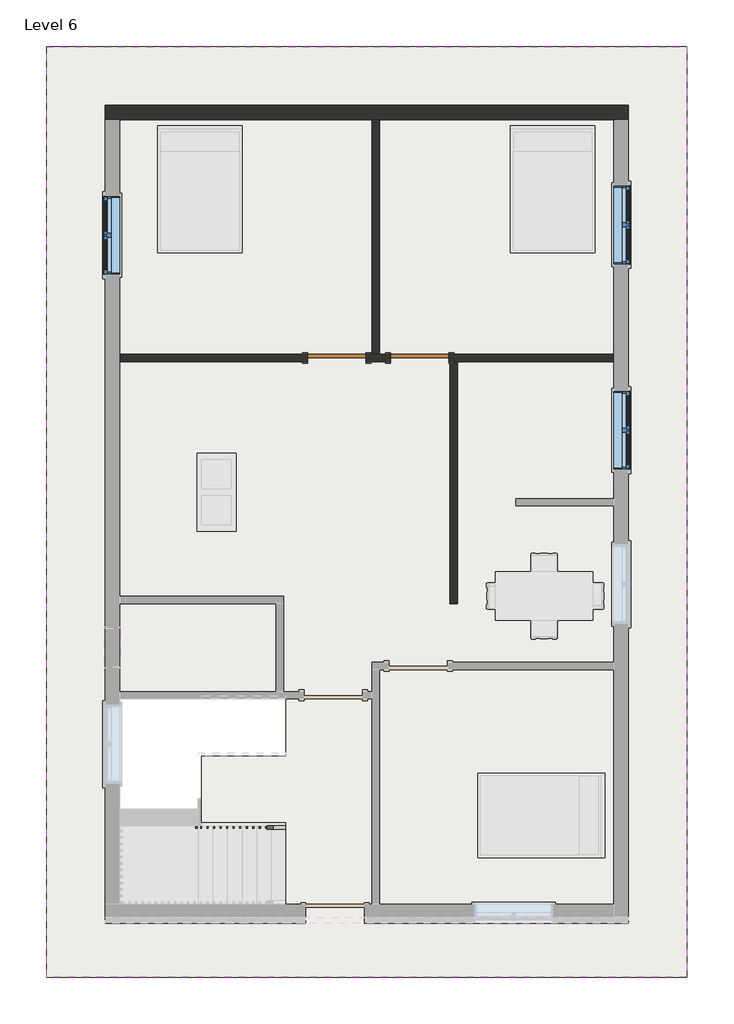
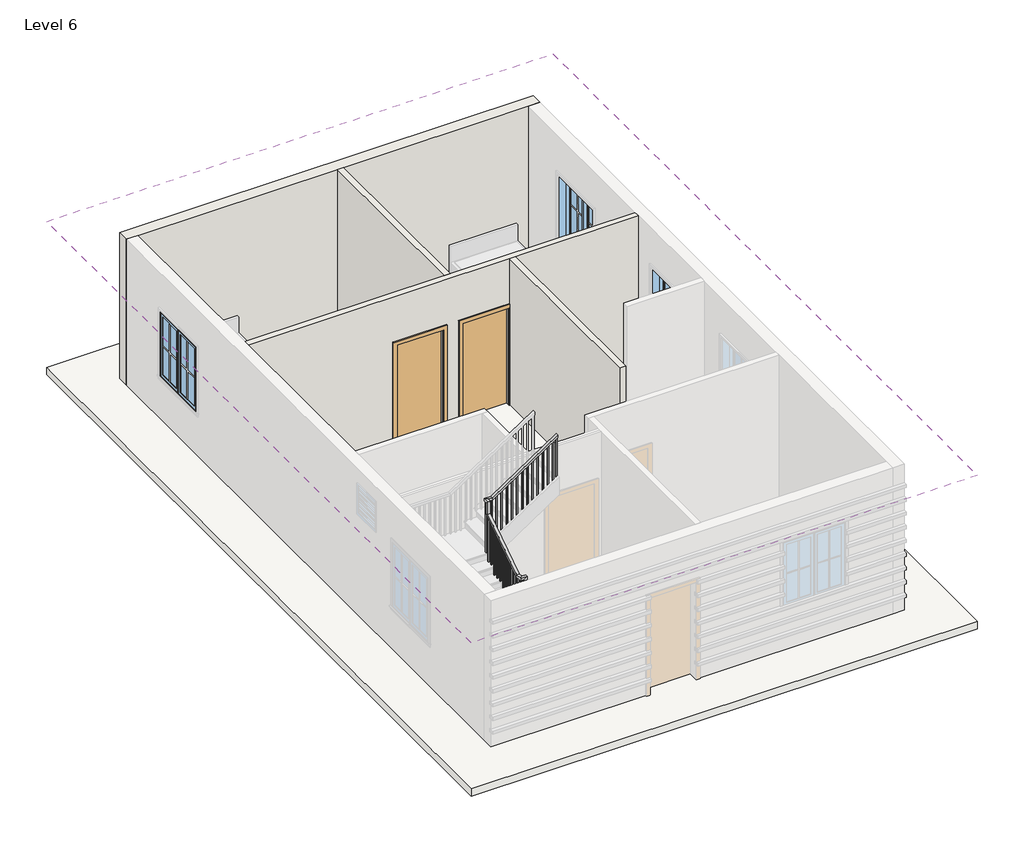
# One storey, part 2 of 3: 4 walls, 3 windows, 2 doors, 2 roofs, 1 railing.
"""IFC4 building model written with IfcOpenShell, lengths in millimetres."""

from ifc_helpers import new_model, si_unit, frame, origin, place, context, project, spatial, polyline, outline, extrude, faceted_brep, transform, mapped, element, save
from components import single_flush_door_3_17d80c48, single_flush_door_3_5e62189b, window_casement_double_window_4_576b2d2c

model = new_model("IFC4")

# Units and contexts
model_context = context("Model", 3, world=origin())
ifc_project = project(units=[si_unit("LENGTHUNIT", "METRE", prefix="MILLI")], contexts=[model_context])

# Site, building, storey
site = spatial("IfcSite", under=ifc_project)
building = spatial("IfcBuilding", under=site)
storey = spatial("IfcBuildingStorey", under=building, Name="Level 6", Elevation=15849.6)

# Doors
placement = place(None, origin())
single_flush_door_3_shape = single_flush_door_3_17d80c48(model_context)
element("IfcDoor", 1, ObjectType="Single-Flush : DOOR 3'", at=placement, inside=storey, context=model_context, shape_type="MappedRepresentation", body=[
    mapped(single_flush_door_3_shape, transform((-1721.4617403, 2133.1073441, 15849.6), x_axis=(1.0, 0.0, 0.0), y_axis=(0.0, 1.0, 0.0), z_axis=(0.0, 0.0, 1.0))),
])
single_flush_door_3_2_shape = single_flush_door_3_5e62189b(model_context)
element("IfcDoor", 2, ObjectType="Single-Flush : DOOR 3'", at=placement, inside=storey, context=model_context, shape_type="MappedRepresentation", body=[
    mapped(single_flush_door_3_2_shape, transform((-426.0617403, 2133.1073441, 15849.6), x_axis=(-1.0, 0.0, 0.0), y_axis=(0.0, -1.0, 0.0), z_axis=(0.0, 0.0, 1.0))),
])

# Railing
element("IfcRailing", 3, ObjectType="Handrail - Rectangular", at=placement, inside=storey, context=model_context, shape_type="SolidModel", body=[
    faceted_brep([(-2515.2117403, -5213.8426559, 16916.4), (-2515.2117403, -5213.8426559, 16855.3459984), (-2515.2117403, -5163.0426559, 16855.3459984), (-2515.2117403, -5163.0426559, 16916.4), (-3810.6117403, -5213.8426559, 17780.0), (-3861.4117403, -5213.8426559, 17752.8126651), (-3861.4117403, -5163.0426559, 17752.8126651), (-3810.6117403, -5163.0426559, 17780.0), (-3810.6117403, -5213.8426559, 18034.0), (-3861.4117403, -5213.8426559, 17983.2), (-3861.4117403, -5163.0426559, 17983.2), (-3810.6117403, -5163.0426559, 18034.0), (-3937.6117403, -5213.8426559, 18034.0), (-3937.6117403, -5213.8426559, 17983.2), (-3886.8117403, -5163.0426559, 17983.2), (-3886.8117403, -5163.0426559, 18034.0), (-3937.6117403, -5086.8426559, 18034.0), (-3937.6117403, -5071.4616535, 17983.2), (-3886.8117403, -5071.4616535, 17983.2), (-3886.8117403, -5086.8426559, 18034.0), (-3937.6117403, -4096.2426559, 18694.4), (-3937.6117403, -4045.4426559, 18667.2126651), (-3886.8117403, -4045.4426559, 18667.2126651), (-3886.8117403, -4096.2426559, 18694.4), (-3937.6117403, -4096.2426559, 18948.4), (-3937.6117403, -4045.4426559, 18897.6), (-3886.8117403, -4045.4426559, 18897.6), (-3886.8117403, -4096.2426559, 18948.4), (-3937.6117403, -3969.2426559, 18948.4), (-3937.6117403, -3969.2426559, 18897.6), (-3886.8117403, -4020.0426559, 18897.6), (-3886.8117403, -4020.0426559, 18948.4), (-3810.6117403, -3969.2426559, 18948.4), (-3795.2307379, -3969.2426559, 18897.6), (-3795.2307379, -4020.0426559, 18897.6), (-3810.6117403, -4020.0426559, 18948.4), (-2515.2117403, -3969.2426559, 19812.0), (-2515.2117403, -4020.0426559, 19812.0), (-2515.2117403, -4020.0426559, 19750.9459984), (-2515.2117403, -3969.2426559, 19750.9459984)], [[[0, 1, 2, 3]], [[1, 0, 4, 5]], [[2, 1, 5, 6]], [[3, 2, 6, 7]], [[0, 3, 7, 4]], [[5, 4, 8, 9]], [[6, 5, 9, 10]], [[7, 6, 10, 11]], [[4, 7, 11, 8]], [[9, 8, 12, 13]], [[10, 9, 13, 14]], [[11, 10, 14, 15]], [[8, 11, 15, 12]], [[13, 12, 16, 17]], [[14, 13, 17, 18]], [[15, 14, 18, 19]], [[12, 15, 19, 16]], [[17, 16, 20, 21]], [[18, 17, 21, 22]], [[19, 18, 22, 23]], [[16, 19, 23, 20]], [[21, 20, 24, 25]], [[22, 21, 25, 26]], [[23, 22, 26, 27]], [[20, 23, 27, 24]], [[25, 24, 28, 29]], [[26, 25, 29, 30]], [[27, 26, 30, 31]], [[24, 27, 31, 28]], [[29, 28, 32, 33]], [[30, 29, 33, 34]], [[31, 30, 34, 35]], [[28, 31, 35, 32]], [[36, 37, 38, 39]], [[33, 32, 36, 39]], [[34, 33, 39, 38]], [[35, 34, 38, 37]], [[32, 35, 37, 36]]]),
    extrude(outline(polyline([(19706.4959984, -2581.8867403), (19693.7959984, -2600.9367403), (18745.2, -2600.9367403), (18745.2, -2581.8867403), (19706.4959984, -2581.8867403)])), frame((0.0, -4004.1676559, 0.0), z_axis=(0.0, 1.0, 0.0), x_axis=(0.0, 0.0, 1.0)), (0.0, 0.0, 1.0), 19.05),
    extrude(outline(polyline([(19638.7626651, -2683.4867403), (19626.0626651, -2702.5367403), (18745.2, -2702.5367403), (18745.2, -2683.4867403), (19638.7626651, -2683.4867403)])), frame((0.0, -4004.1676559, 0.0), z_axis=(0.0, 1.0, 0.0), x_axis=(0.0, 0.0, 1.0)), (0.0, 0.0, 1.0), 19.05),
    extrude(outline(polyline([(19571.0293317, -2785.0867403), (19558.3293317, -2804.1367403), (18592.8, -2804.1367403), (18592.8, -2785.0867403), (19571.0293317, -2785.0867403)])), frame((0.0, -4004.1676559, 0.0), z_axis=(0.0, 1.0, 0.0), x_axis=(0.0, 0.0, 1.0)), (0.0, 0.0, 1.0), 19.05),
    extrude(outline(polyline([(19503.2959984, -2886.6867403), (19490.5959984, -2905.7367403), (18592.8, -2905.7367403), (18592.8, -2886.6867403), (19503.2959984, -2886.6867403)])), frame((0.0, -4004.1676559, 0.0), z_axis=(0.0, 1.0, 0.0), x_axis=(0.0, 0.0, 1.0)), (0.0, 0.0, 1.0), 19.05),
    extrude(outline(polyline([(19435.5626651, -2988.2867403), (19422.8626651, -3007.3367403), (18440.4, -3007.3367403), (18440.4, -2988.2867403), (19435.5626651, -2988.2867403)])), frame((0.0, -4004.1676559, 0.0), z_axis=(0.0, 1.0, 0.0), x_axis=(0.0, 0.0, 1.0)), (0.0, 0.0, 1.0), 19.05),
    extrude(outline(polyline([(19367.8293317, -3089.8867403), (19355.1293317, -3108.9367403), (18440.4, -3108.9367403), (18440.4, -3089.8867403), (19367.8293317, -3089.8867403)])), frame((0.0, -4004.1676559, 0.0), z_axis=(0.0, 1.0, 0.0), x_axis=(0.0, 0.0, 1.0)), (0.0, 0.0, 1.0), 19.05),
    extrude(outline(polyline([(19300.0959984, -3191.4867403), (19287.3959984, -3210.5367403), (18440.4, -3210.5367403), (18440.4, -3191.4867403), (19300.0959984, -3191.4867403)])), frame((0.0, -4004.1676559, 0.0), z_axis=(0.0, 1.0, 0.0), x_axis=(0.0, 0.0, 1.0)), (0.0, 0.0, 1.0), 19.05),
    extrude(outline(polyline([(19232.3626651, -3293.0867403), (19219.6626651, -3312.1367403), (18288.0, -3312.1367403), (18288.0, -3293.0867403), (19232.3626651, -3293.0867403)])), frame((0.0, -4004.1676559, 0.0), z_axis=(0.0, 1.0, 0.0), x_axis=(0.0, 0.0, 1.0)), (0.0, 0.0, 1.0), 19.05),
    extrude(outline(polyline([(19164.6293317, -3394.6867403), (19151.9293317, -3413.7367403), (18288.0, -3413.7367403), (18288.0, -3394.6867403), (19164.6293317, -3394.6867403)])), frame((0.0, -4004.1676559, 0.0), z_axis=(0.0, 1.0, 0.0), x_axis=(0.0, 0.0, 1.0)), (0.0, 0.0, 1.0), 19.05),
    extrude(outline(polyline([(19096.8959984, -3496.2867403), (19084.1959984, -3515.3367403), (18135.6, -3515.3367403), (18135.6, -3496.2867403), (19096.8959984, -3496.2867403)])), frame((0.0, -4004.1676559, 0.0), z_axis=(0.0, 1.0, 0.0), x_axis=(0.0, 0.0, 1.0)), (0.0, 0.0, 1.0), 19.05),
    extrude(outline(polyline([(19029.1626651, -3597.8867403), (19016.4626651, -3616.9367403), (18135.6, -3616.9367403), (18135.6, -3597.8867403), (19029.1626651, -3597.8867403)])), frame((0.0, -4004.1676559, 0.0), z_axis=(0.0, 1.0, 0.0), x_axis=(0.0, 0.0, 1.0)), (0.0, 0.0, 1.0), 19.05),
    extrude(outline(polyline([(18961.4293317, -3699.4867403), (18948.7293317, -3718.5367403), (17983.2, -3718.5367403), (17983.2, -3699.4867403), (18961.4293317, -3699.4867403)])), frame((0.0, -4004.1676559, 0.0), z_axis=(0.0, 1.0, 0.0), x_axis=(0.0, 0.0, 1.0)), (0.0, 0.0, 1.0), 19.05),
    extrude(outline(polyline([(18893.6959984, -3801.0867403), (18880.9959984, -3820.1367403), (17983.2, -3820.1367403), (17983.2, -3801.0867403), (18893.6959984, -3801.0867403)])), frame((0.0, -4004.1676559, 0.0), z_axis=(0.0, 1.0, 0.0), x_axis=(0.0, 0.0, 1.0)), (0.0, 0.0, 1.0), 19.05),
    extrude(outline(polyline([(-3902.6867403, -4080.3676559), (-3921.7367403, -4080.3676559), (-3921.7367403, -4061.3176559), (-3902.6867403, -4061.3176559), (-3902.6867403, -4080.3676559)])), frame((0.0, 0.0, 17678.4), z_axis=(0.0, 0.0, 1.0), x_axis=(1.0, 0.0, 0.0)), (0.0, 0.0, 1.0), 1219.2),
    extrude(outline(polyline([(-4181.9676559, 18576.1959984), (-4162.9176559, 18588.8959984), (-4162.9176559, 17678.4), (-4181.9676559, 17678.4), (-4181.9676559, 18576.1959984)])), frame((-3921.7367403, 0.0, 0.0), z_axis=(1.0, 0.0, 0.0), x_axis=(0.0, 1.0, 0.0)), (0.0, 0.0, 1.0), 19.05),
    extrude(outline(polyline([(-4283.5676559, 18508.4626651), (-4264.5176559, 18521.1626651), (-4264.5176559, 17526.0), (-4283.5676559, 17526.0), (-4283.5676559, 18508.4626651)])), frame((-3921.7367403, 0.0, 0.0), z_axis=(1.0, 0.0, 0.0), x_axis=(0.0, 1.0, 0.0)), (0.0, 0.0, 1.0), 19.05),
    extrude(outline(polyline([(-4385.1676559, 18440.7293317), (-4366.1176559, 18453.4293317), (-4366.1176559, 17526.0), (-4385.1676559, 17526.0), (-4385.1676559, 18440.7293317)])), frame((-3921.7367403, 0.0, 0.0), z_axis=(1.0, 0.0, 0.0), x_axis=(0.0, 1.0, 0.0)), (0.0, 0.0, 1.0), 19.05),
    extrude(outline(polyline([(-4486.7676559, 18372.9959984), (-4467.7176559, 18385.6959984), (-4467.7176559, 17526.0), (-4486.7676559, 17526.0), (-4486.7676559, 18372.9959984)])), frame((-3921.7367403, 0.0, 0.0), z_axis=(1.0, 0.0, 0.0), x_axis=(0.0, 1.0, 0.0)), (0.0, 0.0, 1.0), 19.05),
    extrude(outline(polyline([(-4588.3676559, 18305.2626651), (-4569.3176559, 18317.9626651), (-4569.3176559, 17373.6), (-4588.3676559, 17373.6), (-4588.3676559, 18305.2626651)])), frame((-3921.7367403, 0.0, 0.0), z_axis=(1.0, 0.0, 0.0), x_axis=(0.0, 1.0, 0.0)), (0.0, 0.0, 1.0), 19.05),
    extrude(outline(polyline([(-4689.9676559, 18237.5293317), (-4670.9176559, 18250.2293317), (-4670.9176559, 17373.6), (-4689.9676559, 17373.6), (-4689.9676559, 18237.5293317)])), frame((-3921.7367403, 0.0, 0.0), z_axis=(1.0, 0.0, 0.0), x_axis=(0.0, 1.0, 0.0)), (0.0, 0.0, 1.0), 19.05),
    extrude(outline(polyline([(-4791.5676559, 18169.7959984), (-4772.5176559, 18182.4959984), (-4772.5176559, 17221.2), (-4791.5676559, 17221.2), (-4791.5676559, 18169.7959984)])), frame((-3921.7367403, 0.0, 0.0), z_axis=(1.0, 0.0, 0.0), x_axis=(0.0, 1.0, 0.0)), (0.0, 0.0, 1.0), 19.05),
    extrude(outline(polyline([(-4893.1676559, 18102.0626651), (-4874.1176559, 18114.7626651), (-4874.1176559, 17221.2), (-4893.1676559, 17221.2), (-4893.1676559, 18102.0626651)])), frame((-3921.7367403, 0.0, 0.0), z_axis=(1.0, 0.0, 0.0), x_axis=(0.0, 1.0, 0.0)), (0.0, 0.0, 1.0), 19.05),
    extrude(outline(polyline([(-4994.7676559, 18034.3293317), (-4975.7176559, 18047.0293317), (-4975.7176559, 17068.8), (-4994.7676559, 17068.8), (-4994.7676559, 18034.3293317)])), frame((-3921.7367403, 0.0, 0.0), z_axis=(1.0, 0.0, 0.0), x_axis=(0.0, 1.0, 0.0)), (0.0, 0.0, 1.0), 19.05),
    extrude(outline(polyline([(-5096.3676559, 17966.5959984), (-5077.3176559, 17979.2959984), (-5077.3176559, 17068.8), (-5096.3676559, 17068.8), (-5096.3676559, 17966.5959984)])), frame((-3921.7367403, 0.0, 0.0), z_axis=(1.0, 0.0, 0.0), x_axis=(0.0, 1.0, 0.0)), (0.0, 0.0, 1.0), 19.05),
    extrude(outline(polyline([(-3826.4867403, -5178.9176559), (-3826.4867403, -5197.9676559), (-3845.5367403, -5197.9676559), (-3845.5367403, -5178.9176559), (-3826.4867403, -5178.9176559)])), frame((0.0, 0.0, 16764.0), z_axis=(0.0, 0.0, 1.0), x_axis=(1.0, 0.0, 0.0)), (0.0, 0.0, 1.0), 1219.2),
    extrude(outline(polyline([(17661.7959984, -3724.8867403), (17674.4959984, -3743.9367403), (16764.0, -3743.9367403), (16764.0, -3724.8867403), (17661.7959984, -3724.8867403)])), frame((0.0, -5197.9676559, 0.0), z_axis=(0.0, 1.0, 0.0), x_axis=(0.0, 0.0, 1.0)), (0.0, 0.0, 1.0), 19.05),
    extrude(outline(polyline([(17594.0626651, -3623.2867403), (17606.7626651, -3642.3367403), (16611.6, -3642.3367403), (16611.6, -3623.2867403), (17594.0626651, -3623.2867403)])), frame((0.0, -5197.9676559, 0.0), z_axis=(0.0, 1.0, 0.0), x_axis=(0.0, 0.0, 1.0)), (0.0, 0.0, 1.0), 19.05),
    extrude(outline(polyline([(17526.3293317, -3521.6867403), (17539.0293317, -3540.7367403), (16611.6, -3540.7367403), (16611.6, -3521.6867403), (17526.3293317, -3521.6867403)])), frame((0.0, -5197.9676559, 0.0), z_axis=(0.0, 1.0, 0.0), x_axis=(0.0, 0.0, 1.0)), (0.0, 0.0, 1.0), 19.05),
    extrude(outline(polyline([(17458.5959984, -3420.0867403), (17471.2959984, -3439.1367403), (16611.6, -3439.1367403), (16611.6, -3420.0867403), (17458.5959984, -3420.0867403)])), frame((0.0, -5197.9676559, 0.0), z_axis=(0.0, 1.0, 0.0), x_axis=(0.0, 0.0, 1.0)), (0.0, 0.0, 1.0), 19.05),
    extrude(outline(polyline([(17390.8626651, -3318.4867403), (17403.5626651, -3337.5367403), (16459.2, -3337.5367403), (16459.2, -3318.4867403), (17390.8626651, -3318.4867403)])), frame((0.0, -5197.9676559, 0.0), z_axis=(0.0, 1.0, 0.0), x_axis=(0.0, 0.0, 1.0)), (0.0, 0.0, 1.0), 19.05),
    extrude(outline(polyline([(17323.1293317, -3216.8867403), (17335.8293317, -3235.9367403), (16459.2, -3235.9367403), (16459.2, -3216.8867403), (17323.1293317, -3216.8867403)])), frame((0.0, -5197.9676559, 0.0), z_axis=(0.0, 1.0, 0.0), x_axis=(0.0, 0.0, 1.0)), (0.0, 0.0, 1.0), 19.05),
    extrude(outline(polyline([(17255.3959984, -3115.2867403), (17268.0959984, -3134.3367403), (16306.8, -3134.3367403), (16306.8, -3115.2867403), (17255.3959984, -3115.2867403)])), frame((0.0, -5197.9676559, 0.0), z_axis=(0.0, 1.0, 0.0), x_axis=(0.0, 0.0, 1.0)), (0.0, 0.0, 1.0), 19.05),
    extrude(outline(polyline([(17187.6626651, -3013.6867403), (17200.3626651, -3032.7367403), (16306.8, -3032.7367403), (16306.8, -3013.6867403), (17187.6626651, -3013.6867403)])), frame((0.0, -5197.9676559, 0.0), z_axis=(0.0, 1.0, 0.0), x_axis=(0.0, 0.0, 1.0)), (0.0, 0.0, 1.0), 19.05),
    extrude(outline(polyline([(17119.9293317, -2912.0867403), (17132.6293317, -2931.1367403), (16154.4, -2931.1367403), (16154.4, -2912.0867403), (17119.9293317, -2912.0867403)])), frame((0.0, -5197.9676559, 0.0), z_axis=(0.0, 1.0, 0.0), x_axis=(0.0, 0.0, 1.0)), (0.0, 0.0, 1.0), 19.05),
    extrude(outline(polyline([(17052.1959984, -2810.4867403), (17064.8959984, -2829.5367403), (16154.4, -2829.5367403), (16154.4, -2810.4867403), (17052.1959984, -2810.4867403)])), frame((0.0, -5197.9676559, 0.0), z_axis=(0.0, 1.0, 0.0), x_axis=(0.0, 0.0, 1.0)), (0.0, 0.0, 1.0), 19.05),
    extrude(outline(polyline([(16984.4626651, -2708.8867403), (16997.1626651, -2727.9367403), (16002.0, -2727.9367403), (16002.0, -2708.8867403), (16984.4626651, -2708.8867403)])), frame((0.0, -5197.9676559, 0.0), z_axis=(0.0, 1.0, 0.0), x_axis=(0.0, 0.0, 1.0)), (0.0, 0.0, 1.0), 19.05),
    extrude(outline(polyline([(16916.7293317, -2607.2867403), (16929.4293317, -2626.3367403), (16002.0, -2626.3367403), (16002.0, -2607.2867403), (16916.7293317, -2607.2867403)])), frame((0.0, -5197.9676559, 0.0), z_axis=(0.0, 1.0, 0.0), x_axis=(0.0, 0.0, 1.0)), (0.0, 0.0, 1.0), 19.05),
    extrude(outline(polyline([(-3902.6867403, -4004.1676559), (-3921.7367403, -4004.1676559), (-3921.7367403, -3985.1176559), (-3902.6867403, -3985.1176559), (-3902.6867403, -4004.1676559)])), frame((0.0, 0.0, 17830.8), z_axis=(0.0, 0.0, 1.0), x_axis=(1.0, 0.0, 0.0)), (0.0, 0.0, 1.0), 1066.8),
    extrude(outline(polyline([(-3902.6867403, -5178.9176559), (-3902.6867403, -5197.9676559), (-3921.7367403, -5197.9676559), (-3921.7367403, -5178.9176559), (-3902.6867403, -5178.9176559)])), frame((0.0, 0.0, 16916.4), z_axis=(0.0, 0.0, 1.0), x_axis=(1.0, 0.0, 0.0)), (0.0, 0.0, 1.0), 1066.8),
    extrude(outline(polyline([(19750.9459984, -2515.2117403), (19738.2459984, -2534.2617403), (18745.2, -2534.2617403), (18745.2, -2515.2117403), (19750.9459984, -2515.2117403)])), frame((0.0, -4004.1676559, 0.0), z_axis=(0.0, 1.0, 0.0), x_axis=(0.0, 0.0, 1.0)), (0.0, 0.0, 1.0), 19.05),
    extrude(outline(polyline([(16855.3459984, -2515.2117403), (16868.0459984, -2534.2617403), (16002.0, -2534.2617403), (16002.0, -2515.2117403), (16855.3459984, -2515.2117403)])), frame((0.0, -5197.9676559, 0.0), z_axis=(0.0, 1.0, 0.0), x_axis=(0.0, 0.0, 1.0)), (0.0, 0.0, 1.0), 19.05),
])

# Roofs
element("IfcRoof", 4, ObjectType="ROOF 6\"", at=placement, inside=storey, context=model_context, shape_type="SweptSolid", body=[
    extrude(outline(polyline([(-6249.0117403, -7525.2426559), (-6249.0117403, 6990.8573441), (3745.8882597, 6990.8573441), (3745.8882597, -7525.2426559), (-6249.0117403, -7525.2426559)]), holes=[polyline([(-5156.8117403, -3131.0426559), (-5156.8117403, -6433.0426559), (-2515.2117403, -6433.0426559), (-2515.2117403, -5112.2426559), (-3836.0117403, -5112.2426559), (-3836.0117403, -4070.8426559), (-2515.2117403, -4070.8426559), (-2515.2117403, -3131.0426559), (-5156.8117403, -3131.0426559)])]), frame((0.0, 0.0, 15697.2), z_axis=(0.0, 0.0, 1.0), x_axis=(1.0, 0.0, 0.0)), (0.0, 0.0, 1.0), 152.4),
])
element("IfcRoof", 5, ObjectType="ROOF 6\"", at=placement, inside=storey, context=model_context, shape_type="SweptSolid", body=[
    extrude(outline(polyline([(-6249.0117403, -7525.2426559), (-6249.0117403, 6990.8573441), (3745.8882597, 6990.8573441), (3745.8882597, -7525.2426559), (-6249.0117403, -7525.2426559)]), holes=[polyline([(-5156.8117403, -3131.0426559), (-5156.8117403, -6433.0426559), (-2515.2117403, -6433.0426559), (-2515.2117403, -5112.2426559), (-3836.0117403, -5112.2426559), (-3836.0117403, -4070.8426559), (-2515.2117403, -4070.8426559), (-2515.2117403, -3131.0426559), (-5156.8117403, -3131.0426559)])]), frame((0.0, 0.0, 18897.6), z_axis=(0.0, 0.0, 1.0), x_axis=(1.0, 0.0, 0.0)), (0.0, 0.0, 1.0), 152.4),
])

# Walls
element("IfcWall", 6, ObjectType="ALL 4.5\"", at=placement, inside=storey, context=model_context, shape_type="Brep", body=[
    faceted_brep([(-1264.2617403, 2075.9573441, 15849.6), (-883.2617403, 2075.9573441, 15849.6), (-883.2617403, 2075.9573441, 17881.6), (31.1382597, 2075.9573441, 17881.6), (31.1382597, 2075.9573441, 15849.6), (50.1882597, 2075.9573441, 15849.6), (164.4882597, 2075.9573441, 15849.6), (2602.8882597, 2075.9573441, 15849.6), (2602.8882597, 2075.9573441, 18897.6), (164.4882597, 2075.9573441, 18897.6), (50.1882597, 2075.9573441, 18897.6), (-5106.0117403, 2075.9573441, 18897.6), (-5106.0117403, 2075.9573441, 15849.6), (-2178.6617403, 2075.9573441, 15849.6), (-2178.6617403, 2075.9573441, 17881.6), (-1264.2617403, 2075.9573441, 17881.6), (-883.2617403, 2190.2573441, 17881.6), (-883.2617403, 2190.2573441, 15849.6), (-1054.7117403, 2190.2573441, 15849.6), (-1169.0117403, 2190.2573441, 15849.6), (-1264.2617403, 2190.2573441, 15849.6), (-1264.2617403, 2190.2573441, 17881.6), (-2178.6617403, 2190.2573441, 17881.6), (-2178.6617403, 2190.2573441, 15849.6), (-5106.0117403, 2190.2573441, 15849.6), (-5106.0117403, 2190.2573441, 18897.6), (-1169.0117403, 2190.2573441, 18897.6), (-1054.7117403, 2190.2573441, 18897.6), (2602.8882597, 2190.2573441, 18897.6), (2602.8882597, 2190.2573441, 15849.6), (31.1382597, 2190.2573441, 15849.6), (31.1382597, 2190.2573441, 17881.6)], [[[0, 1, 2, 3, 4, 5, 6, 7, 8, 9, 10, 11, 12, 13, 14, 15]], [[16, 17, 18, 19, 20, 21, 22, 23, 24, 25, 26, 27, 28, 29, 30, 31]], [[13, 12, 24, 23]], [[30, 29, 7, 6, 5, 4]], [[20, 19, 18, 17, 1, 0]], [[8, 7, 29, 28]], [[12, 11, 25, 24]], [[21, 20, 0, 15]], [[22, 21, 15, 14]], [[23, 22, 14, 13]], [[2, 1, 17, 16]], [[3, 2, 16, 31]], [[4, 3, 31, 30]], [[11, 10, 9, 8, 28, 27, 26, 25]]]),
])
element("IfcWall", 7, ObjectType="ALL 4.5\"", at=placement, inside=storey, context=model_context, shape_type="SweptSolid", body=[
    extrude(outline(polyline([(50.1882597, -1695.9426559), (50.1882597, 2075.9573441), (164.4882597, 2075.9573441), (164.4882597, -1695.9426559), (50.1882597, -1695.9426559)])), frame((0.0, 0.0, 15849.6), z_axis=(0.0, 0.0, 1.0), x_axis=(1.0, 0.0, 0.0)), (0.0, 0.0, 1.0), 3048.0),
])
element("IfcWall", 8, ObjectType="ALL 4.5\"", at=placement, inside=storey, context=model_context, shape_type="SweptSolid", body=[
    extrude(outline(polyline([(-1169.0117403, 2190.2573441), (-1169.0117403, 5847.8573441), (-1054.7117403, 5847.8573441), (-1054.7117403, 2190.2573441), (-1169.0117403, 2190.2573441)])), frame((0.0, 0.0, 15849.6), z_axis=(0.0, 0.0, 1.0), x_axis=(1.0, 0.0, 0.0)), (0.0, 0.0, 1.0), 3048.0),
])
element("IfcWall", 9, ObjectType="WALL 9\"", at=placement, inside=storey, context=model_context, shape_type="Brep", body=[
    faceted_brep([(-5334.6117403, 5847.8573441, 15849.6), (-5106.0117403, 5847.8573441, 15849.6), (-1169.0117403, 5847.8573441, 15849.6), (-1054.7117403, 5847.8573441, 15849.6), (2602.8882597, 5847.8573441, 15849.6), (2831.4882597, 5847.8573441, 15849.6), (2831.4882597, 5847.8573441, 18897.6), (2602.8882597, 5847.8573441, 18897.6), (-1054.7117403, 5847.8573441, 18897.6), (-1169.0117403, 5847.8573441, 18897.6), (-5106.0117403, 5847.8573441, 18897.6), (-5334.6117403, 5847.8573441, 18897.6), (-5334.6117403, 6076.4573441, 15849.6), (-5334.6117403, 6076.4573441, 18897.6), (2831.4882597, 6076.4573441, 18897.6), (2831.4882597, 6076.4573441, 15849.6)], [[[0, 1, 2, 3, 4, 5, 6, 7, 8, 9, 10, 11]], [[12, 13, 14, 15]], [[5, 4, 3, 2, 1, 0, 12, 15]], [[6, 5, 15, 14]], [[0, 11, 13, 12]], [[11, 10, 9, 8, 7, 6, 14, 13]]]),
])

# Windows
window_casement_double_window_4_shape = window_casement_double_window_4_576b2d2c(model_context)
element("IfcWindow", 10, ObjectType="Window-Casement-Double : WINDOW 4'", at=placement, inside=storey, context=model_context, shape_type="MappedRepresentation", body=[
    mapped(window_casement_double_window_4_shape, transform((-5220.3117403, 4047.6323441, 15849.6), x_axis=(0.0, 1.0, 0.0), y_axis=(-1.0, 0.0, 0.0), z_axis=(0.0, 0.0, 1.0))),
])
element("IfcWindow", 11, ObjectType="Window-Casement-Double : WINDOW 4'", at=placement, inside=storey, context=model_context, shape_type="MappedRepresentation", body=[
    mapped(window_casement_double_window_4_shape, transform((2717.1882597, 4209.5573441, 15849.6), x_axis=(0.0, -1.0, 0.0), y_axis=(1.0, 0.0, 0.0), z_axis=(0.0, 0.0, 1.0))),
])
element("IfcWindow", 12, ObjectType="Window-Casement-Double : WINDOW 4'", at=placement, inside=storey, context=model_context, shape_type="MappedRepresentation", body=[
    mapped(window_casement_double_window_4_shape, transform((2717.1882597, 1009.1573441, 15849.6), x_axis=(0.0, -1.0, 0.0), y_axis=(1.0, 0.0, 0.0), z_axis=(0.0, 0.0, 1.0))),
])

save(model, "model.ifc")

# Revit data of these elements
# Type "Single-Flush : DOOR 3'"
#   Type Mark = "8"
#   Construction Type Id = "MDOOR"
#   Assembly Code = "C1020"
#   Analytic Construction = "Metal"
#   Thickness = 0' - 2"
#   Heat Transfer Coefficient (U) = 0.651978 BTU/(h·ft²·°F)
#   Height = 6' - 8"
#   Trim Projection Ext = 0' - 1"
#   Trim Projection Int = 0' - 1"
#   Trim Width = 0' - 3"
#   Width = 3' - 0"
#   Define Thermal Properties by = 1
#   Door Material = Door - Panel
#   Frame Material = Door - Frame
#   Visual Light Transmittance = 0
#   Solar Heat Gain Coefficient = 0
#   Function = (empty or 0)
#   Wall Closure = (empty or 0)
# Type "Handrail - Rectangular"
#   Assembly Code = "C2010400"
#   built-in parameter 1008612 = 0.0416667 (stored number, unit not read)
#   built-in parameter 1008611 = 0.0416667 (stored number, unit not read)
#   built-in parameter 1008609 = 0.333333 (stored number, unit not read)
#   built-in parameter 1008604 = 0.166667 (stored number, unit not read)
#   built-in parameter 1008603 = 0.166667 (stored number, unit not read)
#   Railing Height = 3' - 0"
#   built-in parameter 1008630 = 2
#   built-in parameter 1008610 = 2
#   built-in parameter 1008618 = Baluster - Square : 3/4"
# Type "ROOF 6\""
#   Assembly Code = "B1020"
#   Layers, outside or top first: 0' - 6" no material (function 1)
# Type "ALL 4.5\""
#   Assembly Code = "B2010"
#   Layers, outside or top first: 0' - 4 1/2" no material (function 1)
# Type "WALL 9\""
#   Assembly Code = "B2010"
#   Layers, outside or top first: 0' - 9" "Carpet (1)" (function 1)
# Type "Window-Casement-Double : WINDOW 4'"
#   Type Mark = "18"
#   Fire Rating = "0.5h"
#   Assembly Code = "B2020100"
#   Analytic Construction = "Double glazing - domestic"
#   Frame Extension [instance default] = 0' - 0 1/4"
#   Window Inset [instance default] = 0' - 0"
#   Wall Thickness [instance default] = 0' - 6"
#   Interior Wall Closure [instance default] = 0' - 2 1/4"
#   Half Width = 2' - 0"
#   Visual Light Transmittance = 0.81
#   Thermal Resistance (R) = 1.8146 (h·ft²·°F)/BTU
#   Solar Heat Gain Coefficient = 0.76
#   Rough Width = 4' - 0 1/2"
#   Rough Height = 4' - 5 1/2"
#   Height = 4' - 5"
#   Heat Transfer Coefficient (U) = 0.5511 BTU/(h·ft²·°F)
#   Exterior Wall Closure [instance default] = 0' - 1 1/4"
#   Extension Jamb [instance default] = 0' - 2 1/4"
#   Default Sill Height = 3' - 0"
#   Width = 4' - 0"
#   Muntin Visibility = yes
#   Interior Trim Visibility [instance default] = yes
#   Exterior Trim Visibility [instance default] = yes
#   Extension Jamb Visibility [instance default] = yes
#   Interior Trim Material = Wood - Stained
#   Muntin Pattern = Muntin Pattern_2x2 : Muntin Pattern_2x2
#   Interior Trim = Trim-Window-Interior-Flat : Picture Frame
#   Interior Frame Material = Wood - Stained
#   Glass Panel Material = Glass
#   Exterior Trim Material = Clad - White
#   Exterior Trim = Trim-Window-Exterior-Flat : with Sill
#   Exterior Frame Material = Clad - White
#   Wall Closure = (empty or 0)
# Elements 1, 2 (IfcDoor, "Single-Flush : DOOR 3'")
#   Phase Created = New Construction
#   Materials on its faces: "Door - Frame", "Door - Panel"
# Element 3 (IfcRailing, "Handrail - Rectangular")
#   Phase Created = New Construction
#   Materials on its faces: "Clad - White"
# Element 4 (IfcRoof, "ROOF 6\"")
#   built-in parameter 1001705 = 52 (stored number, unit not read)
#   built-in parameter 1001701 = -0.5 (stored number, unit not read)
#   built-in parameter 1001710 = 33615
#   Phase Created = New Construction
#   Materials on its faces: "Clad - White", "Default Roof", "Softwood, Lumber"
# Element 5 (IfcRoof, "ROOF 6\"")
#   built-in parameter 1001705 = 62.5 (stored number, unit not read)
#   built-in parameter 1001701 = 10 (stored number, unit not read)
#   built-in parameter 1001710 = 33615
#   Phase Created = New Construction
#   Materials on its faces: "Clad - White", "Default Roof", "Softwood, Lumber"
# Elements 6, 7, 8 (IfcWall, "ALL 4.5\"")
#   Top Offset = 0' - 0"
#   Base Offset = 0' - 0"
#   Unconnected Height = 10' - 0"
#   wall height = 10' - 0"
#   Phase Created = New Construction
#   Base Constraint = Level 6
#   Materials on its faces: "Default Wall"
# Element 9 (IfcWall, "WALL 9\"")
#   Top Offset = 0' - 0"
#   Base Offset = 0' - 0"
#   Unconnected Height = 10' - 0"
#   wall height = 10' - 0"
#   Phase Created = New Construction
#   Base Constraint = Level 6
#   Materials on its faces: "Carpet (1)", "Wood - Stained"
# Element 10 (IfcWindow, "Window-Casement-Double : WINDOW 4'")
#   Mark = "37"
#   Window Inset = 0' - 0"
#   Interior Wall Closure = 0' - 2 1/4"
#   Frame Extension = 0' - 0 1/4"
#   Exterior Wall Closure = 0' - 1 1/4"
#   Interior Trim Visibility = yes
#   Exterior Trim Visibility = yes
#   Phase Created = New Construction
#   Materials on its faces: "Wood - Stained", "Glass", "Clad - White"
# Element 11 (IfcWindow, "Window-Casement-Double : WINDOW 4'")
#   Mark = "38"
#   Window Inset = 0' - 0"
#   Interior Wall Closure = 0' - 2 1/4"
#   Frame Extension = 0' - 0 1/4"
#   Exterior Wall Closure = 0' - 1 1/4"
#   Interior Trim Visibility = yes
#   Exterior Trim Visibility = yes
#   Phase Created = New Construction
#   Materials on its faces: "Wood - Stained", "Glass", "Clad - White"
# Element 12 (IfcWindow, "Window-Casement-Double : WINDOW 4'")
#   Mark = "39"
#   Window Inset = 0' - 0"
#   Interior Wall Closure = 0' - 2 1/4"
#   Frame Extension = 0' - 0 1/4"
#   Exterior Wall Closure = 0' - 1 1/4"
#   Interior Trim Visibility = yes
#   Exterior Trim Visibility = yes
#   Phase Created = New Construction
#   Materials on its faces: "Wood - Stained", "Glass", "Clad - White"
# Materials
#   "Door - Panel": class "Wood", colour RGB 210 159 95, transparency 0, Cost = 0
#   "Door - Frame": colour RGB 118 70 51, transparency 0, Cost = 0
#   "Carpet (1)": class "Carpet", colour RGB 124 80 67, transparency 0, Description = "Interior finish", Cost = 0
#   "Wood - Stained": class "Wood", colour RGB 224 178 126, transparency 0, Cost = 0
#   "Glass": class "Glass", colour RGB 0 128 192, transparency 0.75, Description = "Soda Lime Glass", Cost = 0
#   "Clad - White": class "Wood", colour RGB 242 242 238, transparency 0, Cost = 0
#   "Default Roof": colour RGB 88 101 114, transparency 0, Cost = 0
#   "Softwood, Lumber": class "Wood", colour RGB 223 192 134, transparency 0, Description = "Pinus Echinata", Cost = 0
#   "Default Wall": colour RGB 128 128 128, transparency 0, Cost = 0
